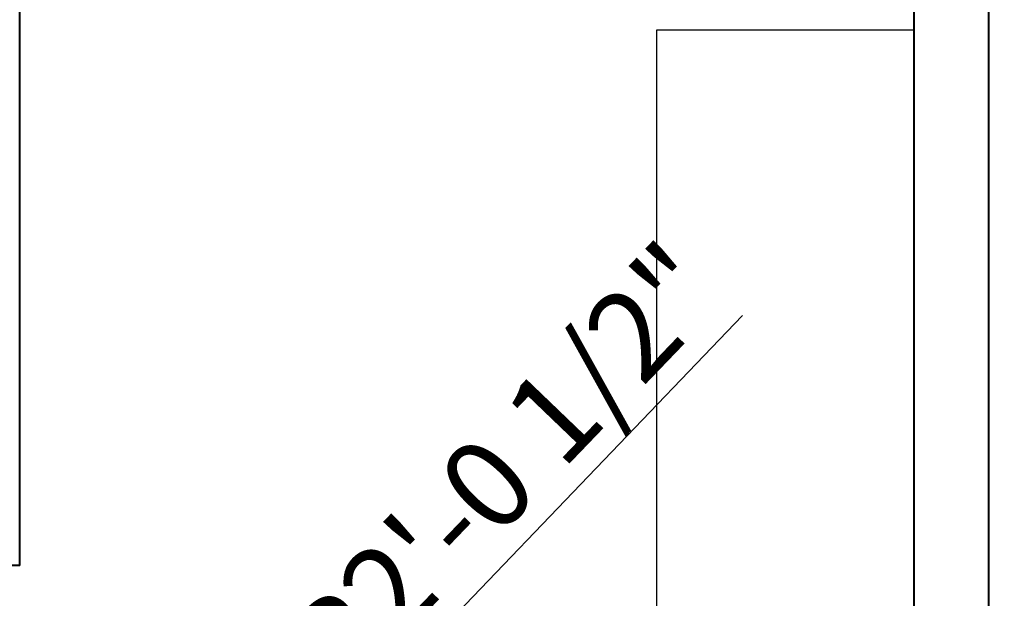
# Model space of a CAD drawing. Units: inches. Extents: x 459864 to 460310, y 324185 to 324787.
# Tile 68 of 112: x 460061 to 460127, y 324321 to 324360. Entities that reach past the tile are written whole.
import ezdxf

# ---------------------------------------------------------------- set-up
doc = ezdxf.new("R2010")
doc.units = ezdxf.units.IN
for name, color, linetype, lineweight in [('A-ANNO-DIMS', 2, 'Continuous', 18), ('A-FLOR-CASE', 8, 'Continuous', 25), ('A-WALL', 7, 'Continuous', 40)]:
    doc.layers.add(name, color=color, linetype=linetype, lineweight=lineweight)
doc.styles.get("Standard").update_dxf_attribs({"font": 'arial.ttf'})
doc.dimstyles.new('ISO-25', dxfattribs={"dimtxt": 6, "dimasz": 2.5, "dimexe": 1.25, "dimexo": 0.625, "dimtad": 1, "dimdec": 1, "dimlunit": 3, "dimtxsty": 'Standard', "dimcen": 2.5, "dimadec": 0, "dimazin": 0, "dimtfac": 1, "dimtdec": 1, "dimtmove": 0, "dimatfit": 3, "dimfxl": 1, "dimarcsym": 0})

# ---------------------------------------------------------------- blocks, each defined once
blk = doc.blocks.new('*D28')
at = {"layer": 'A-ANNO-DIMS', "color": 0, "lineweight": -2, "transparency": 16777216}
for p, q in [((460148.65, 324370.7), (460136.025, 324370.7)), ((460137.275, 324368.2), (460137.275, 324293.2)), ((460148.65, 324290.7), (460136.025, 324290.7)), ((460137.275, 324290.7), (460137.275, 324198.69))]:
    blk.add_line(p, q, dxfattribs=at)
at = {"layer": 'A-ANNO-DIMS', "color": 0, "transparency": 16777216}
for points in [[(460136.858, 324368.2), (460137.692, 324368.2), (460137.275, 324370.7)], [(460136.858, 324293.2), (460137.692, 324293.2), (460137.275, 324290.7)]]:
    blk.add_solid(points, dxfattribs=at)
at = {"layer": 'Defpoints', "color": 0, "transparency": 16777216}
for p in [(460149.275, 324370.7), (460137.275, 324290.7), (460149.275, 324290.7)]:
    blk.add_point(p, dxfattribs=at)
at = {"layer": 'A-ANNO-DIMS', "color": 0, "transparency": 16777216, "insert": (460133.363, 324243.445), "char_height": 6, "attachment_point": 5, "rotation": 90}
blk.add_mtext('QUEEN BED 6\'-8" TYP.', dxfattribs=at)
blk = doc.blocks.new('*D69')
at = {"layer": 'A-ANNO-DIMS', "color": 0, "lineweight": -2, "transparency": 16777216}
for p, q in [((460055.99, 324376.483), (459874.965, 324376.483)), ((459876.215, 324373.983), (459876.215, 324285.983)), ((460060.49, 324283.483), (459874.965, 324283.483))]:
    blk.add_line(p, q, dxfattribs=at)
at = {"layer": 'A-ANNO-DIMS', "color": 0, "transparency": 16777216}
for points in [[(459875.798, 324373.983), (459876.632, 324373.983), (459876.215, 324376.483)], [(459875.798, 324285.983), (459876.632, 324285.983), (459876.215, 324283.483)]]:
    blk.add_solid(points, dxfattribs=at)
at = {"layer": 'Defpoints', "color": 0, "transparency": 16777216}
for p in [(460056.615, 324376.483), (459876.215, 324283.483), (460061.115, 324283.483)]:
    blk.add_point(p, dxfattribs=at)
at = {"layer": 'A-ANNO-DIMS', "color": 0, "transparency": 16777216, "insert": (459872.526, 324329.983), "char_height": 6, "attachment_point": 5, "rotation": 90}
blk.add_mtext('7\'-9"', dxfattribs=at)
blk = doc.blocks.new('*D73')
at = {"layer": 'A-ANNO-DIMS', "color": 0, "lineweight": -2, "transparency": 16777216}
for p, q in [((460109.617, 324339.904), (460082.316, 324311.465)), ((460063.615, 324291.983), (460080.585, 324309.661))]:
    blk.add_line(p, q, dxfattribs=at)
at = {"layer": 'A-ANNO-DIMS', "color": 0, "transparency": 16777216}
blk.add_solid([(460082.016, 324311.753), (460082.617, 324311.176), (460080.585, 324309.661)], dxfattribs=at)
at = {"layer": 'Defpoints', "color": 0, "transparency": 16777216}
for p in [(460080.585, 324309.661), (460063.615, 324291.983)]:
    blk.add_point(p, dxfattribs=at)
at = {"layer": 'A-ANNO-DIMS', "color": 0, "transparency": 16777216, "insert": (460094.144, 324329.167), "char_height": 6, "attachment_point": 5, "rotation": 46.17012}
blk.add_mtext('R2\'-0 1/2"', dxfattribs=at)

msp = doc.modelspace()

# ---------------------------------------------------------------- linework, layer by layer
at = {"layer": 'A-FLOR-CASE'}
for p, q in [((460121.115, 324359.05), (460103.847, 324359.05)), ((460103.847, 324359.05), (460103.847, 324311.967))]:
    msp.add_line(p, q, dxfattribs=at)
at = {"layer": 'A-WALL'}
for p, q in [((460121.115, 324399.05), (460121.115, 324283.483)), ((460126.115, 324399.05), (460126.115, 324283.483)), ((460061.115, 324323.126), (460061.115, 324380.983)), ((460061.115, 324323.126), (460056.615, 324323.126))]:
    msp.add_line(p, q, dxfattribs=at)

# ---------------------------------------------------------------- dimensions: what is measured, and where the dimension line sits
at = {"layer": 'A-ANNO-DIMS'}
dim = msp.add_linear_dim(base=(459876.215, 324283.483), p1=(460056.615, 324376.483), p2=(460061.115, 324283.483), angle=90, dimstyle='ISO-25', override={"dimdec": 1, "dimlfac": 1, "dimrnd": 0, "dimzin": 1, "dimdsep": 46, "dimlunit": 4, "dimfrac": 2}, dxfattribs=at)
dim.commit()
dim.dimension.update_dxf_attribs({"geometry": '*D69', "text_midpoint": (459872.526, 324329.983)})
dim = msp.add_linear_dim(base=(460137.275, 324290.7), p1=(460149.275, 324370.7), p2=(460149.275, 324290.7), angle=270, text='QUEEN BED <> TYP.', dimstyle='ISO-25', override={"dimdec": 1, "dimlfac": 1, "dimrnd": 0, "dimzin": 1, "dimdsep": 46, "dimlunit": 4, "dimfrac": 2}, dxfattribs=at)
dim.commit()
dim.dimension.update_dxf_attribs({"geometry": '*D28', "text_midpoint": (460133.363, 324243.445)})
dim = msp.add_radius_dim(center=(460063.615, 324291.983), mpoint=(460080.585, 324309.661), dimstyle='ISO-25', override={"dimdec": 1, "dimlfac": 1, "dimrnd": 0, "dimzin": 1, "dimdsep": 46, "dimlunit": 4, "dimfrac": 2}, dxfattribs=at)
dim.commit()
dim.dimension.update_dxf_attribs({"geometry": '*D73', "text_midpoint": (460094.144, 324329.167)})

doc.saveas('drawing.dxf')
